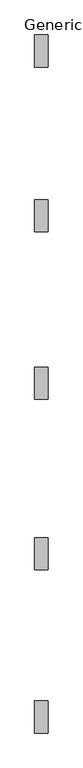
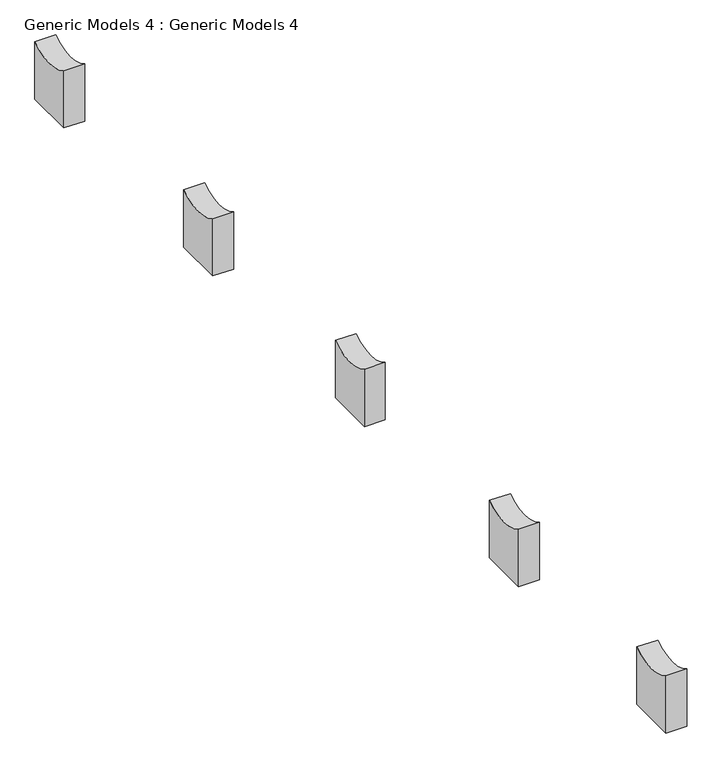
"""IFC4 building model written with IfcOpenShell, lengths in millimetres: proxy geometry, Generic Models 4 : Generic Models 4."""

from ifc_helpers import new_model, si_unit, point, frame, frame_2d, origin, place, context, project, spatial, polyline, circle_curve, trimmed, segment, composite_curve, outline, extrude, source, transform, mapped, element, save


def generic_models_4_generic_models_4_b5ce0ccc(model_context):
    return source(origin(), model_context, "Body", "SweptSolid", [
        extrude(outline(composite_curve([segment(polyline([(7939.9582203, 587.7593504), (7939.9582203, 1476.7593504)]), True, "CONTINUOUS"), segment(trimmed(circle_curve(frame_2d((8309.1582762, 2022.4493373)), 658.8522163), [point((7939.9582203, 1476.7593504))], [point((8678.358332, 1476.7593504))], True, "CARTESIAN"), True, "CONTINUOUS"), segment(polyline([(8678.358332, 1476.7593504), (8678.358332, 587.7593504), (7939.9582203, 587.7593504)]), True, "CONTINUOUS")], self_intersect=False)), frame((8003.5487756, 0.0, 0.0), z_axis=(1.0, 0.0, 0.0), x_axis=(0.0, 1.0, 0.0)), (0.0, 0.0, 1.0), 304.8),
        extrude(outline(composite_curve([segment(polyline([(4150.5957203, 587.7593504), (4150.5957203, 1476.7593504)]), True, "CONTINUOUS"), segment(trimmed(circle_curve(frame_2d((4519.7957762, 2022.4493373)), 658.8522163), [point((4150.5957203, 1476.7593504))], [point((4888.995832, 1476.7593504))], True, "CARTESIAN"), True, "CONTINUOUS"), segment(polyline([(4888.995832, 1476.7593504), (4888.995832, 587.7593504), (4150.5957203, 587.7593504)]), True, "CONTINUOUS")], self_intersect=False)), frame((8003.5487756, 0.0, 0.0), z_axis=(1.0, 0.0, 0.0), x_axis=(0.0, 1.0, 0.0)), (0.0, 0.0, 1.0), 304.8),
        extrude(outline(composite_curve([segment(polyline([(293.5660328, 587.7593504), (293.5660328, 1476.7593504)]), True, "CONTINUOUS"), segment(trimmed(circle_curve(frame_2d((662.7660887, 2022.4493373)), 658.8522163), [point((293.5660328, 1476.7593504))], [point((1031.9661445, 1476.7593504))], True, "CARTESIAN"), True, "CONTINUOUS"), segment(polyline([(1031.9661445, 1476.7593504), (1031.9661445, 587.7593504), (293.5660328, 587.7593504)]), True, "CONTINUOUS")], self_intersect=False)), frame((8003.5487756, 0.0, 0.0), z_axis=(1.0, 0.0, 0.0), x_axis=(0.0, 1.0, 0.0)), (0.0, 0.0, 1.0), 304.8),
        extrude(outline(composite_curve([segment(polyline([(-3631.1308422, 483.6747029), (-3631.1308422, 1372.6747029)]), True, "CONTINUOUS"), segment(trimmed(circle_curve(frame_2d((-3261.9307863, 1918.3646897)), 658.8522163), [point((-3631.1308422, 1372.6747029))], [point((-2892.7307305, 1372.6747029))], True, "CARTESIAN"), True, "CONTINUOUS"), segment(polyline([(-2892.7307305, 1372.6747029), (-2892.7307305, 483.6747029), (-3631.1308422, 483.6747029)]), True, "CONTINUOUS")], self_intersect=False)), frame((8003.5487756, 0.0, 0.0), z_axis=(1.0, 0.0, 0.0), x_axis=(0.0, 1.0, 0.0)), (0.0, 0.0, 1.0), 304.8),
        extrude(outline(composite_curve([segment(polyline([(-7383.690273, 483.6747029), (-7383.690273, 1372.6747029)]), True, "CONTINUOUS"), segment(trimmed(circle_curve(frame_2d((-7014.4902172, 1918.3646897)), 658.8522163), [point((-7383.690273, 1372.6747029))], [point((-6645.2901613, 1372.6747029))], True, "CARTESIAN"), True, "CONTINUOUS"), segment(polyline([(-6645.2901613, 1372.6747029), (-6645.2901613, 483.6747029), (-7383.690273, 483.6747029)]), True, "CONTINUOUS")], self_intersect=False)), frame((8003.5487756, 0.0, 0.0), z_axis=(1.0, 0.0, 0.0), x_axis=(0.0, 1.0, 0.0)), (0.0, 0.0, 1.0), 304.8),
    ])


if __name__ == "__main__":
    model = new_model("IFC4")
    model_context = context("Model", 3, world=origin())
    ifc_project = project(units=[si_unit("LENGTHUNIT", "METRE", prefix="MILLI")], contexts=[model_context])
    site = spatial("IfcSite", under=ifc_project)
    building = spatial("IfcBuilding", under=site)
    placement = place(None, origin())
    generic_models_4_generic_models_4_shape = generic_models_4_generic_models_4_b5ce0ccc(model_context)
    element("IfcBuildingElementProxy", 1, Name="Generic Models 4 : Generic Models 4", ObjectType="Generic Models 4 : Generic Models 4", at=placement, inside=building, context=model_context, shape_type="MappedRepresentation", body=[
        mapped(generic_models_4_generic_models_4_shape, transform((0.0, 0.0, 0.0), x_axis=(1.0, 0.0, 0.0), y_axis=(0.0, 1.0, 0.0), z_axis=(0.0, 0.0, 1.0))),
    ])
    save(model, "model.ifc")

# Revit data of these elements
# Element 1 (IfcBuildingElementProxy, "Generic Models 4 : Generic Models 4")
#   Materials on its faces: "Parking Stripe"
# Materials
#   "Parking Stripe": class "Paint", colour RGB 250 250 91, transparency 0, Cost = 0
